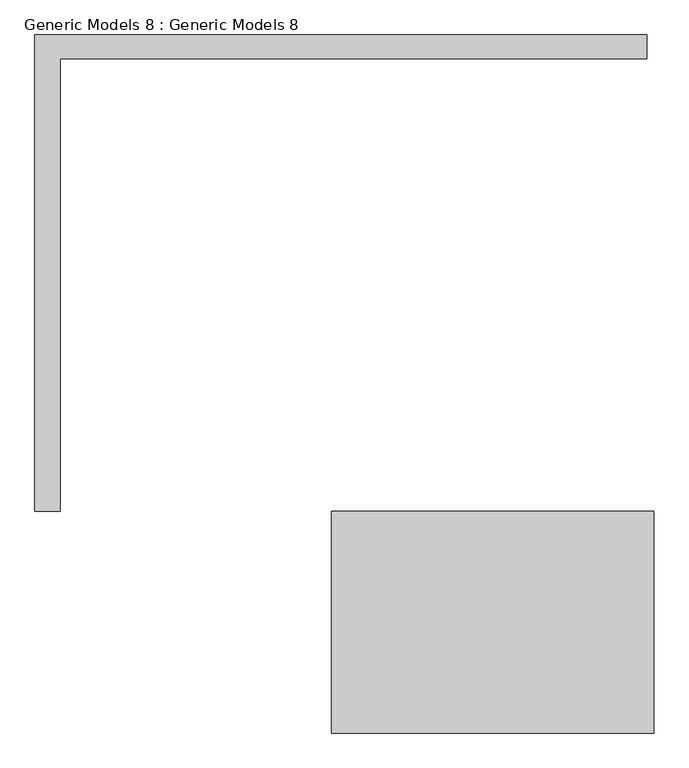
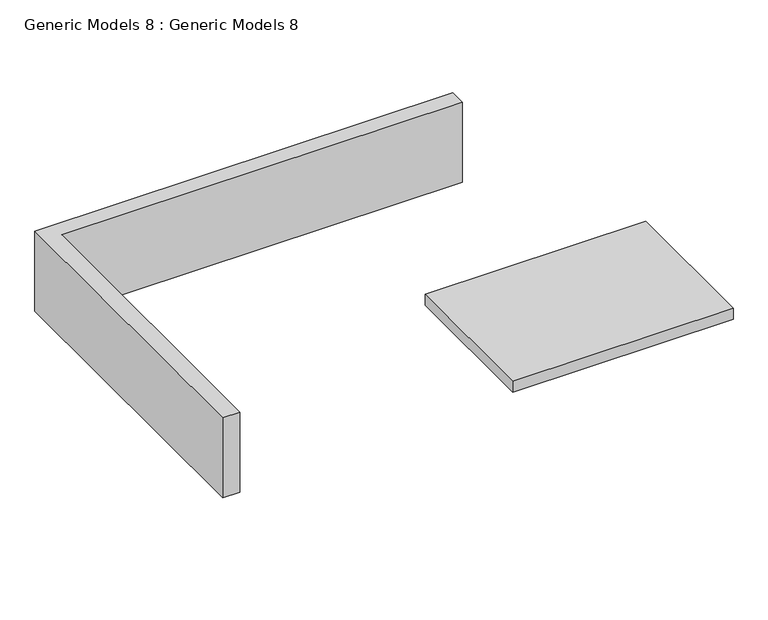
"""IFC4 building model written with IfcOpenShell, lengths in millimetres: proxy geometry, Generic Models 8 : Generic Models 8."""

from ifc_helpers import new_model, si_unit, frame, origin, place, context, project, spatial, polyline, outline, extrude, source, transform, mapped, element, save


def generic_models_8_generic_models_8_3e5e579e(model_context):
    return source(origin(), model_context, "Body", "SweptSolid", [
        extrude(outline(polyline([(-4980.5321088, -5738.2962979), (-4980.5321088, -9642.8158046), (-10657.4321088, -9642.8158046), (-10657.4321088, -5738.2962979), (-4980.5321088, -5738.2962979)])), frame((0.0, 0.0, 9813.4676011), z_axis=(0.0, 0.0, 1.0), x_axis=(1.0, 0.0, 0.0)), (0.0, 0.0, 1.0), 301.2403051),
        extrude(outline(polyline([(-15432.7587428, 2220.0531596), (-15432.7587428, -5738.2962979), (-15877.1321088, -5738.2962979), (-15877.1321088, 2639.1531596), (-5107.5321088, 2639.1531596), (-5107.5321088, 2220.0531596), (-15432.7587428, 2220.0531596)])), frame((0.0, 0.0, 6400.8), z_axis=(0.0, 0.0, 1.0), x_axis=(1.0, 0.0, 0.0)), (0.0, 0.0, 1.0), 2178.143726),
    ])


if __name__ == "__main__":
    model = new_model("IFC4")
    model_context = context("Model", 3, world=origin())
    ifc_project = project(units=[si_unit("LENGTHUNIT", "METRE", prefix="MILLI")], contexts=[model_context])
    site = spatial("IfcSite", under=ifc_project)
    building = spatial("IfcBuilding", under=site)
    placement = place(None, origin())
    generic_models_8_generic_models_8_shape = generic_models_8_generic_models_8_3e5e579e(model_context)
    element("IfcBuildingElementProxy", 1, Name="Generic Models 8 : Generic Models 8", ObjectType="Generic Models 8 : Generic Models 8", at=placement, inside=building, context=model_context, shape_type="MappedRepresentation", body=[
        mapped(generic_models_8_generic_models_8_shape, transform((0.0, 0.0, 0.0), x_axis=(1.0, 0.0, 0.0), y_axis=(0.0, 1.0, 0.0), z_axis=(0.0, 0.0, 1.0))),
    ])
    save(model, "model.ifc")
